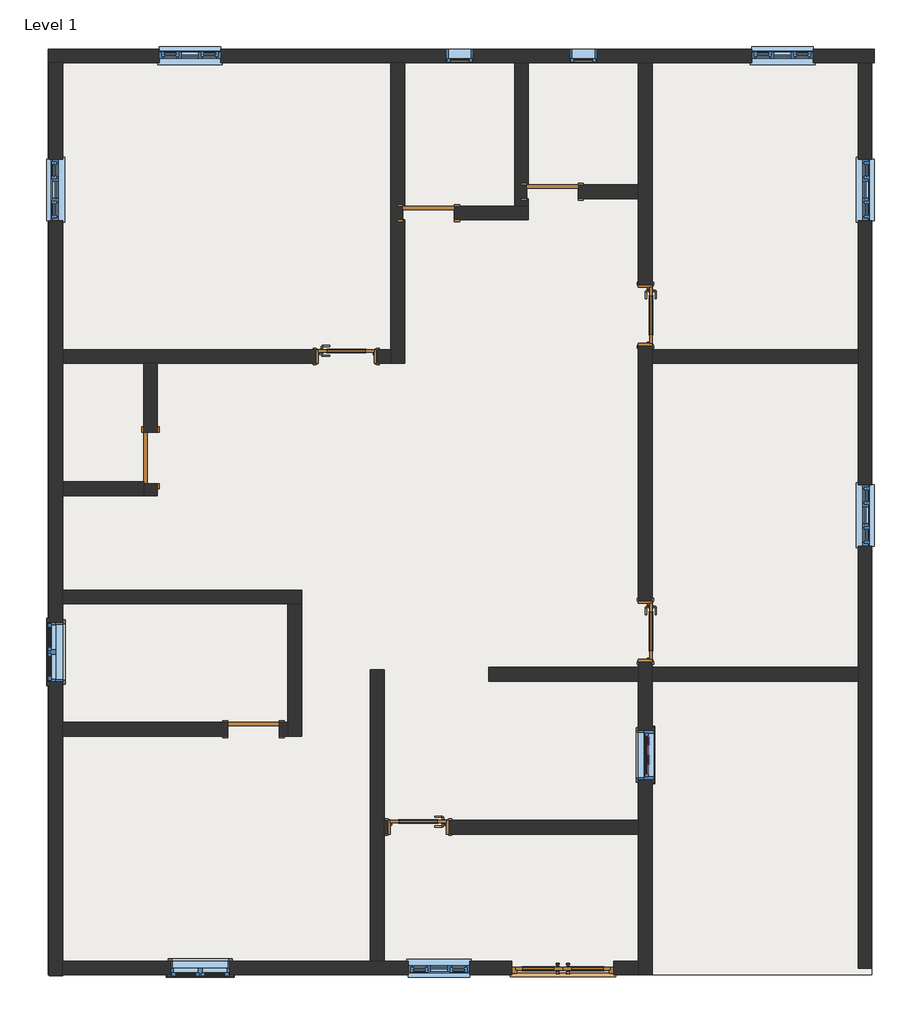
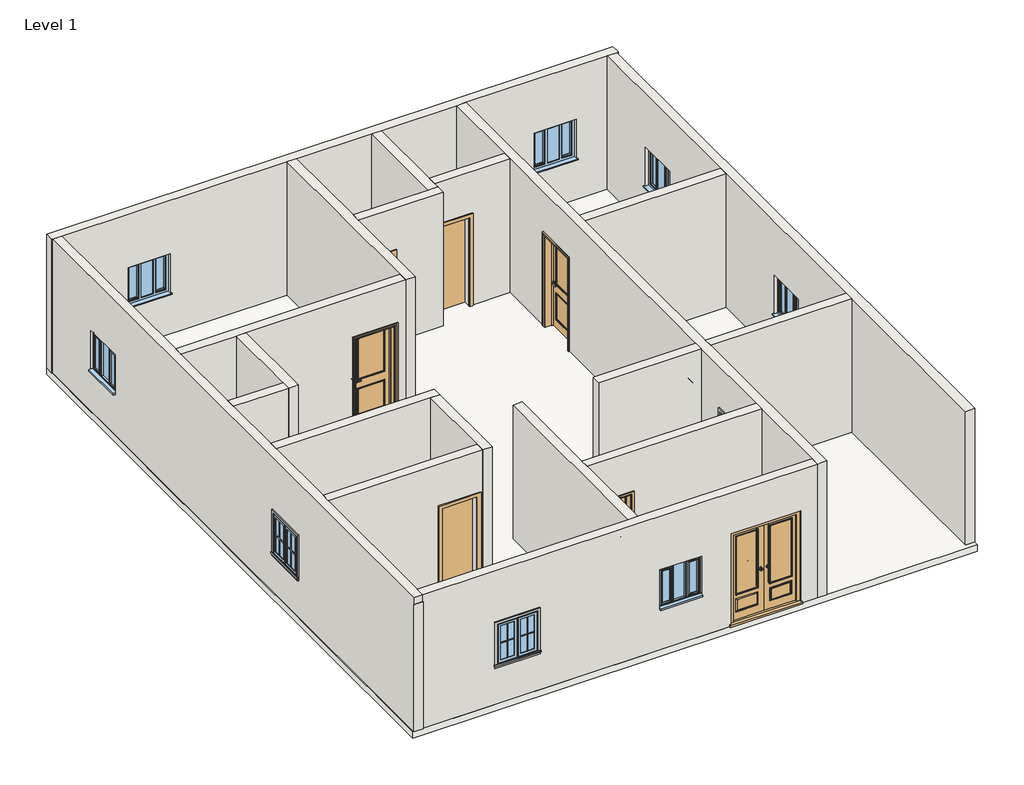
# One storey, incomplete: 19 walls, 12 proxies, 11 windows, 9 doors, 1 slab.
"""IFC4 building model written with IfcOpenShell, lengths in millimetres."""

from ifc_helpers import new_model, si_unit, frame, origin, origin_with_axes, place, context, project, spatial, polyline, outline, extrude, faceted_brep, transform, mapped, element, save
from components import muntin_pattern_2x2_muntin_pattern_2x2_b3fe6957, muntin_pattern_2x2_muntin_pattern_2x2_3e0ecaf2, muntin_pattern_2x2_muntin_pattern_2x2_5f474966, trim_window_exterior_flat_with_sill_41619996, trim_window_exterior_flat_with_sill_68241f6a, trim_window_interior_flat_picture_frame_51c85655, trim_window_interior_flat_picture_frame_d3d93820, doors_extdbl_w_glazing_bars_2_1510x2110mm_e5cd3545, doors_extdbl_w_glazing_bars_2_1510x2110mm_b3535315, doors_intsgl_w_transome_910x2110mm_1071bad6, doors_intsgl_w_transome_910x2110mm_0d7ac49b, door_fadea3f2, door_53b1b562, window_085f26e1, window_c29befe5, window_4d695ea9, windows_tpl_plain_910x910mm_84e79c20

model = new_model("IFC4")

# Units and contexts
model_context = context("Model", 3, world=origin())
ifc_project = project(units=[si_unit("LENGTHUNIT", "METRE", prefix="MILLI")], contexts=[model_context])

# Site, building, storey
site = spatial("IfcSite", under=ifc_project)
building = spatial("IfcBuilding", under=site)
storey = spatial("IfcBuildingStorey", under=building, Name="Level 1", Elevation=0.0)

# Proxies
placement = place(None, origin())
muntin_pattern_2x2_muntin_pattern_2x2_shape = muntin_pattern_2x2_muntin_pattern_2x2_b3fe6957(model_context)
element("IfcBuildingElementProxy", 1, Name="Muntin Pattern_2x2 : Muntin Pattern_2x2", ObjectType="Muntin Pattern_2x2 : Muntin Pattern_2x2", at=placement, inside=storey, context=model_context, shape_type="MappedRepresentation", body=[
    mapped(muntin_pattern_2x2_muntin_pattern_2x2_shape, transform((-4444.3565281, -6259.9254533, 984.25), x_axis=(-1.0, 0.0, 0.0), y_axis=(0.0, -1.0, 0.0), z_axis=(0.0, 0.0, 1.0))),
])
element("IfcBuildingElementProxy", 2, Name="Muntin Pattern_2x2 : Muntin Pattern_2x2", ObjectType="Muntin Pattern_2x2 : Muntin Pattern_2x2", at=placement, inside=storey, context=model_context, shape_type="MappedRepresentation", body=[
    mapped(muntin_pattern_2x2_muntin_pattern_2x2_shape, transform((-6884.3440281, -1708.5629533, 984.25), x_axis=(0.0, 1.0, 0.0), y_axis=(-1.0, 0.0, 0.0), z_axis=(0.0, 0.0, 1.0))),
])
muntin_pattern_2x2_muntin_pattern_2x2_2_shape = muntin_pattern_2x2_muntin_pattern_2x2_3e0ecaf2(model_context)
element("IfcBuildingElementProxy", 3, Name="Muntin Pattern_2x2 : Muntin Pattern_2x2", ObjectType="Muntin Pattern_2x2 : Muntin Pattern_2x2", at=placement, inside=storey, context=model_context, shape_type="MappedRepresentation", body=[
    mapped(muntin_pattern_2x2_muntin_pattern_2x2_2_shape, transform((-4872.9815281, -6259.9254533, 984.25), x_axis=(1.0, 0.0, 0.0), y_axis=(0.0, 1.0, 0.0), z_axis=(0.0, 0.0, 1.0))),
])
element("IfcBuildingElementProxy", 4, Name="Muntin Pattern_2x2 : Muntin Pattern_2x2", ObjectType="Muntin Pattern_2x2 : Muntin Pattern_2x2", at=placement, inside=storey, context=model_context, shape_type="MappedRepresentation", body=[
    mapped(muntin_pattern_2x2_muntin_pattern_2x2_2_shape, transform((-6884.3440281, -1279.9379533, 984.25), x_axis=(0.0, -1.0, 0.0), y_axis=(1.0, 0.0, 0.0), z_axis=(0.0, 0.0, 1.0))),
])
muntin_pattern_2x2_muntin_pattern_2x2_3_shape = muntin_pattern_2x2_muntin_pattern_2x2_5f474966(model_context)
element("IfcBuildingElementProxy", 5, Name="Muntin Pattern_2x2 : Muntin Pattern_2x2", ObjectType="Muntin Pattern_2x2 : Muntin Pattern_2x2", at=placement, inside=storey, context=model_context, shape_type="MappedRepresentation", body=[
    mapped(muntin_pattern_2x2_muntin_pattern_2x2_3_shape, transform((1989.809459, -3018.2504533, 1520.825), x_axis=(0.0, -1.0, 0.0), y_axis=(1.0, 0.0, 0.0), z_axis=(0.0, 0.0, 1.0))),
])
element("IfcBuildingElementProxy", 6, Name="Muntin Pattern_2x2 : Muntin Pattern_2x2", ObjectType="Muntin Pattern_2x2 : Muntin Pattern_2x2", at=placement, inside=storey, context=model_context, shape_type="MappedRepresentation", body=[
    mapped(muntin_pattern_2x2_muntin_pattern_2x2_3_shape, transform((1945.359459, -3018.2504533, 990.6), x_axis=(0.0, -1.0, 0.0), y_axis=(1.0, 0.0, 0.0), z_axis=(0.0, 0.0, 1.0))),
])
trim_window_exterior_flat_with_sill_shape = trim_window_exterior_flat_with_sill_41619996(model_context)
element("IfcBuildingElementProxy", 7, Name="Trim-Window-Exterior-Flat : with Sill", ObjectType="Trim-Window-Exterior-Flat : with Sill", at=placement, inside=storey, context=model_context, shape_type="MappedRepresentation", body=[
    mapped(trim_window_exterior_flat_with_sill_shape, transform((-4658.6690281, -6269.4504533, 1828.8), x_axis=(1.0, 0.0, 0.0), y_axis=(0.0, 0.0, 1.0), z_axis=(0.0, -1.0, 0.0))),
])
element("IfcBuildingElementProxy", 8, Name="Trim-Window-Exterior-Flat : with Sill", ObjectType="Trim-Window-Exterior-Flat : with Sill", at=placement, inside=storey, context=model_context, shape_type="MappedRepresentation", body=[
    mapped(trim_window_exterior_flat_with_sill_shape, transform((-6893.8690281, -1494.2504533, 1828.8), x_axis=(0.0, -1.0, 0.0), y_axis=(0.0, 0.0, 1.0), z_axis=(-1.0, 0.0, 0.0))),
])
trim_window_exterior_flat_with_sill_2_shape = trim_window_exterior_flat_with_sill_68241f6a(model_context)
element("IfcBuildingElementProxy", 9, Name="Trim-Window-Exterior-Flat : with Sill", ObjectType="Trim-Window-Exterior-Flat : with Sill", at=placement, inside=storey, context=model_context, shape_type="MappedRepresentation", body=[
    mapped(trim_window_exterior_flat_with_sill_2_shape, transform((2024.734459, -3018.2504533, 2082.8), x_axis=(0.0, 1.0, 0.0), y_axis=(0.0, 0.0, 1.0), z_axis=(1.0, 0.0, 0.0))),
])
trim_window_interior_flat_picture_frame_shape = trim_window_interior_flat_picture_frame_51c85655(model_context)
element("IfcBuildingElementProxy", 10, Name="Trim-Window-Interior-Flat : Picture Frame", ObjectType="Trim-Window-Interior-Flat : Picture Frame", at=placement, inside=storey, context=model_context, shape_type="MappedRepresentation", body=[
    mapped(trim_window_interior_flat_picture_frame_shape, transform((-4658.6690281, -6066.2504533, 1828.8), x_axis=(-1.0, 0.0, 0.0), y_axis=(0.0, 0.0, 1.0), z_axis=(0.0, 1.0, 0.0))),
])
element("IfcBuildingElementProxy", 11, Name="Trim-Window-Interior-Flat : Picture Frame", ObjectType="Trim-Window-Interior-Flat : Picture Frame", at=placement, inside=storey, context=model_context, shape_type="MappedRepresentation", body=[
    mapped(trim_window_interior_flat_picture_frame_shape, transform((-6690.6690281, -1494.2504533, 1828.8), x_axis=(0.0, 1.0, 0.0), y_axis=(0.0, 0.0, 1.0), z_axis=(1.0, 0.0, 0.0))),
])
trim_window_interior_flat_picture_frame_2_shape = trim_window_interior_flat_picture_frame_d3d93820(model_context)
element("IfcBuildingElementProxy", 12, Name="Trim-Window-Interior-Flat : Picture Frame", ObjectType="Trim-Window-Interior-Flat : Picture Frame", at=placement, inside=storey, context=model_context, shape_type="MappedRepresentation", body=[
    mapped(trim_window_interior_flat_picture_frame_2_shape, transform((1821.534459, -3018.2504533, 2082.8), x_axis=(0.0, -1.0, 0.0), y_axis=(0.0, 0.0, 1.0), z_axis=(-1.0, 0.0, 0.0))),
])

# Doors
doors_extdbl_w_glazing_bars_2_1510x2110mm_shape = doors_extdbl_w_glazing_bars_2_1510x2110mm_e5cd3545(model_context)
doors_extdbl_w_glazing_bars_2_1510x2110mm_2_shape = doors_extdbl_w_glazing_bars_2_1510x2110mm_b3535315(model_context)
element("IfcDoor", 13, ObjectType="Doors_ExtDbl_w-Glazing_Bars_2 : 1510x2110mm", at=placement, inside=storey, context=model_context, shape_type="MappedRepresentation", body=[
    mapped(doors_extdbl_w_glazing_bars_2_1510x2110mm_shape, transform((703.934459, -6167.8504533, 0.0), x_axis=(-1.0, 0.0, 0.0), y_axis=(0.0, -1.0, 0.0), z_axis=(0.0, 0.0, 1.0))),
    mapped(doors_extdbl_w_glazing_bars_2_1510x2110mm_2_shape, transform((703.934459, -6167.8504533, 0.0), x_axis=(-1.0, 0.0, 0.0), y_axis=(0.0, -1.0, 0.0), z_axis=(0.0, 0.0, 1.0))),
])
doors_intsgl_w_transome_910x2110mm_shape = doors_intsgl_w_transome_910x2110mm_1071bad6(model_context)
element("IfcDoor", 14, ObjectType="Doors_IntSgl_w-Transome : 910x2110mm", at=placement, inside=storey, context=model_context, shape_type="MappedRepresentation", body=[
    mapped(doors_intsgl_w_transome_910x2110mm_shape, transform((-1432.8690281, -4085.0504533, 0.0), x_axis=(-1.0, 0.0, 0.0), y_axis=(0.0, -1.0, 0.0), z_axis=(0.0, 0.0, 1.0))),
])
doors_intsgl_w_transome_910x2110mm_2_shape = doors_intsgl_w_transome_910x2110mm_0d7ac49b(model_context)
element("IfcDoor", 15, ObjectType="Doors_IntSgl_w-Transome : 910x2110mm", at=placement, inside=storey, context=model_context, shape_type="MappedRepresentation", body=[
    mapped(doors_intsgl_w_transome_910x2110mm_2_shape, transform((-2499.6690281, 2874.5495467, 0.0), x_axis=(1.0, 0.0, 0.0), y_axis=(0.0, 1.0, 0.0), z_axis=(0.0, 0.0, 1.0))),
])
element("IfcDoor", 16, ObjectType="Doors_IntSgl_w-Transome : 910x2110mm", at=placement, inside=storey, context=model_context, shape_type="MappedRepresentation", body=[
    mapped(doors_intsgl_w_transome_910x2110mm_2_shape, transform((1923.134459, 3484.1495467, 0.0), x_axis=(0.0, -1.0, 0.0), y_axis=(1.0, 0.0, 0.0), z_axis=(0.0, 0.0, 1.0))),
])
element("IfcDoor", 17, ObjectType="Doors_IntSgl_w-Transome : 910x2110mm", at=placement, inside=storey, context=model_context, shape_type="MappedRepresentation", body=[
    mapped(doors_intsgl_w_transome_910x2110mm_2_shape, transform((1923.134459, -1189.4504533, 0.0), x_axis=(0.0, -1.0, 0.0), y_axis=(1.0, 0.0, 0.0), z_axis=(0.0, 0.0, 1.0))),
])
door_shape = door_fadea3f2(model_context)
element("IfcDoor", 18, ObjectType="Single-Flush : 30\" x 80\"", at=placement, inside=storey, context=model_context, shape_type="MappedRepresentation", body=[
    mapped(door_shape, transform((-3871.2690281, -2637.2504533, 0.0), x_axis=(1.0, 0.0, 0.0), y_axis=(0.0, 1.0, 0.0), z_axis=(0.0, 0.0, 1.0))),
])
door_2_shape = door_53b1b562(model_context)
element("IfcDoor", 19, ObjectType="Single-Flush : 30\" x 80\"", at=placement, inside=storey, context=model_context, shape_type="MappedRepresentation", body=[
    mapped(door_2_shape, transform((-5395.2690281, 1375.9495467, 0.0), x_axis=(0.0, -1.0, 0.0), y_axis=(1.0, 0.0, 0.0), z_axis=(0.0, 0.0, 1.0))),
])
element("IfcDoor", 20, ObjectType="Single-Flush : 30\" x 80\"", at=placement, inside=storey, context=model_context, shape_type="MappedRepresentation", body=[
    mapped(door_2_shape, transform((-1280.4690281, 4995.4495467, 0.0), x_axis=(-1.0, 0.0, 0.0), y_axis=(0.0, -1.0, 0.0), z_axis=(0.0, 0.0, 1.0))),
])
element("IfcDoor", 21, ObjectType="Single-Flush : 30\" x 80\"", at=placement, inside=storey, context=model_context, shape_type="MappedRepresentation", body=[
    mapped(door_2_shape, transform((548.3309719, 5312.9495467, 0.0), x_axis=(-1.0, 0.0, 0.0), y_axis=(0.0, -1.0, 0.0), z_axis=(0.0, 0.0, 1.0))),
])

# Slab
element("IfcSlab", 22, ObjectType="Generic - 12\"", at=placement, inside=storey, context=model_context, shape_type="SweptSolid", body=[
    extrude(outline(polyline([(5272.7309719, 7421.1495467), (5272.7309719, -6269.4504533), (-6906.5690281, -6269.4504533), (-6906.5690281, 7421.1495467), (5272.7309719, 7421.1495467)])), frame((0.0, 0.0, -152.4), z_axis=(0.0, 0.0, 1.0), x_axis=(1.0, 0.0, 0.0)), (0.0, 0.0, 1.0), 152.4),
])

# Walls
element("IfcWall", 23, ObjectType="4.5\" p", at=placement, inside=storey, context=model_context, shape_type="Brep", body=[
    faceted_brep([(-1839.2690281, 7217.9495467, 0.0), (-1839.2690281, 2976.1495467, 0.0), (-1839.2690281, 2772.9495467, 0.0), (-1839.2690281, 2772.9495467, 3048.0), (-1839.2690281, 2976.1495467, 3048.0), (-1839.2690281, 7217.9495467, 3048.0), (-1636.0690281, 7217.9495467, 3048.0), (-1636.0690281, 5097.0495467, 3048.0), (-1636.0690281, 4893.8495467, 3048.0), (-1636.0690281, 2772.9495467, 3048.0), (-1636.0690281, 2772.9495467, 0.0), (-1636.0690281, 4893.8495467, 0.0), (-1636.0690281, 4893.8495467, 2032.0), (-1636.0690281, 5097.0495467, 2032.0), (-1636.0690281, 5097.0495467, 0.0), (-1636.0690281, 7217.9495467, 0.0), (-1661.4690281, 5097.0495467, 0.0), (-1661.4690281, 4893.8495467, 0.0), (-1661.4690281, 5097.0495467, 2032.0), (-1661.4690281, 4893.8495467, 2032.0)], [[[0, 1, 2, 3, 4, 5]], [[6, 7, 8, 9, 10, 11, 12, 13, 14, 15]], [[2, 1, 0, 15, 14, 16, 17, 11, 10]], [[5, 4, 3, 9, 8, 7, 6]], [[0, 5, 6, 15]], [[3, 2, 10, 9]], [[18, 16, 14, 13]], [[17, 19, 12, 11]], [[19, 18, 13, 12]], [[16, 18, 19, 17]]]),
])
element("IfcWall", 24, ObjectType="4.5\" p", at=placement, inside=storey, context=model_context, shape_type="Brep", body=[
    faceted_brep([(-1839.2690281, 2772.9495467, 3048.0), (-5293.6690281, 2772.9495467, 3048.0), (-5496.8690281, 2772.9495467, 3048.0), (-6690.6690281, 2772.9495467, 3048.0), (-6690.6690281, 2772.9495467, 0.0), (-5496.8690281, 2772.9495467, 0.0), (-5293.6690281, 2772.9495467, 0.0), (-2954.6690281, 2772.9495467, 0.0), (-2954.6690281, 2772.9495467, 2110.0), (-2044.6690281, 2772.9495467, 2110.0), (-2044.6690281, 2772.9495467, 0.0), (-1839.2690281, 2772.9495467, 0.0), (-6690.6690281, 2976.1495467, 3048.0), (-1839.2690281, 2976.1495467, 3048.0), (-1839.2690281, 2976.1495467, 0.0), (-2044.6690281, 2976.1495467, 0.0), (-2044.6690281, 2976.1495467, 2110.0), (-2954.6690281, 2976.1495467, 2110.0), (-2954.6690281, 2976.1495467, 0.0), (-6690.6690281, 2976.1495467, 0.0)], [[[0, 1, 2, 3, 4, 5, 6, 7, 8, 9, 10, 11]], [[12, 13, 14, 15, 16, 17, 18, 19]], [[4, 19, 18, 7, 6, 5]], [[14, 11, 10, 15]], [[3, 2, 1, 0, 13, 12]], [[0, 11, 14, 13]], [[4, 3, 12, 19]], [[9, 16, 15, 10]], [[16, 9, 8, 17]], [[17, 8, 7, 18]]]),
])
element("IfcWall", 25, ObjectType="4.5\" p", at=placement, inside=storey, context=model_context, shape_type="Brep", body=[
    faceted_brep([(-5496.8690281, 994.9495467, 2032.0), (-5496.8690281, 994.9495467, 0.0), (-5496.8690281, 817.1495467, 0.0), (-5496.8690281, 817.1495467, 3048.0), (-5496.8690281, 1020.3495467, 3048.0), (-5496.8690281, 2772.9495467, 3048.0), (-5496.8690281, 2772.9495467, 0.0), (-5496.8690281, 1756.9495467, 0.0), (-5496.8690281, 1756.9495467, 2032.0), (-5293.6690281, 817.1495467, 0.0), (-5293.6690281, 994.9495467, 0.0), (-5293.6690281, 994.9495467, 2032.0), (-5293.6690281, 1756.9495467, 2032.0), (-5293.6690281, 1756.9495467, 0.0), (-5293.6690281, 2772.9495467, 0.0), (-5293.6690281, 2772.9495467, 3048.0), (-5293.6690281, 817.1495467, 3048.0)], [[[0, 1, 2, 3, 4, 5, 6, 7, 8]], [[9, 10, 11, 12, 13, 14, 15, 16]], [[7, 6, 14, 13]], [[2, 1, 10, 9]], [[5, 4, 3, 16, 15]], [[6, 5, 15, 14]], [[3, 2, 9, 16]], [[11, 10, 1, 0]], [[12, 11, 0, 8]], [[13, 12, 8, 7]]]),
])
element("IfcWall", 26, ObjectType="4.5\" p", at=placement, inside=storey, context=model_context, shape_type="Brep", body=[
    faceted_brep([(-6690.6690281, 817.1495467, 0.0), (-5496.8690281, 817.1495467, 0.0), (-5496.8690281, 817.1495467, 3048.0), (-6690.6690281, 817.1495467, 3048.0), (-6690.6690281, 1020.3495467, 0.0), (-6690.6690281, 1020.3495467, 3048.0), (-5496.8690281, 1020.3495467, 3048.0), (-5496.8690281, 1020.3495467, 0.0), (-5496.8690281, 994.9495467, 0.0)], [[[0, 1, 2, 3]], [[4, 5, 6, 7]], [[1, 0, 4, 7, 8]], [[3, 2, 6, 5]], [[2, 1, 8, 7, 6]], [[0, 3, 5, 4]]]),
])
element("IfcWall", 27, ObjectType="4.5\" p", at=placement, inside=storey, context=model_context, shape_type="Brep", body=[
    faceted_brep([(-6690.6690281, -783.0504533, 0.0), (-3363.2690281, -783.0504533, 0.0), (-3160.0690281, -783.0504533, 0.0), (-3160.0690281, -783.0504533, 3048.0), (-3363.2690281, -783.0504533, 3048.0), (-6690.6690281, -783.0504533, 3048.0), (-6690.6690281, -579.8504533, 0.0), (-6690.6690281, -579.8504533, 3048.0), (-3160.0690281, -579.8504533, 3048.0), (-3160.0690281, -579.8504533, 0.0)], [[[0, 1, 2, 3, 4, 5]], [[6, 7, 8, 9]], [[2, 1, 0, 6, 9]], [[5, 4, 3, 8, 7]], [[0, 5, 7, 6]], [[3, 2, 9, 8]]]),
])
element("IfcWall", 28, ObjectType="4.5\" p", at=placement, inside=storey, context=model_context, shape_type="Brep", body=[
    faceted_brep([(-3363.2690281, -783.0504533, 0.0), (-3363.2690281, -2535.6504533, 0.0), (-3363.2690281, -2738.8504533, 0.0), (-3363.2690281, -2738.8504533, 3048.0), (-3363.2690281, -2535.6504533, 3048.0), (-3363.2690281, -783.0504533, 3048.0), (-3160.0690281, -783.0504533, 0.0), (-3160.0690281, -783.0504533, 3048.0), (-3160.0690281, -2738.8504533, 3048.0), (-3160.0690281, -2738.8504533, 0.0)], [[[0, 1, 2, 3, 4, 5]], [[6, 7, 8, 9]], [[2, 1, 0, 6, 9]], [[5, 4, 3, 8, 7]], [[0, 5, 7, 6]], [[3, 2, 9, 8]]]),
])
element("IfcWall", 29, ObjectType="4.5\" p", at=placement, inside=storey, context=model_context, shape_type="SweptSolid", body=[
    extrude(outline(polyline([(2032.0, -3490.2690281), (0.0, -3490.2690281), (0.0, -3363.2690281), (3048.0, -3363.2690281), (3048.0, -6690.6690281), (0.0, -6690.6690281), (0.0, -4252.2690281), (2032.0, -4252.2690281), (2032.0, -3490.2690281)])), frame((0.0, -2738.8504533, 0.0), z_axis=(0.0, 1.0, 0.0), x_axis=(0.0, 0.0, 1.0)), (0.0, 0.0, 1.0), 203.2),
])
element("IfcWall", 30, ObjectType="4.5\" p", at=placement, inside=storey, context=model_context, shape_type="Brep", body=[
    faceted_brep([(192.7309719, 4893.8495467, 3048.0), (-1636.0690281, 4893.8495467, 3048.0), (-1636.0690281, 4893.8495467, 2032.0), (-899.4690281, 4893.8495467, 2032.0), (-899.4690281, 4893.8495467, 0.0), (192.7309719, 4893.8495467, 0.0), (-1636.0690281, 5097.0495467, 3048.0), (-10.4690281, 5097.0495467, 3048.0), (192.7309719, 5097.0495467, 3048.0), (192.7309719, 5097.0495467, 0.0), (-10.4690281, 5097.0495467, 0.0), (-899.4690281, 5097.0495467, 0.0), (-899.4690281, 5097.0495467, 2032.0), (-1636.0690281, 5097.0495467, 2032.0)], [[[0, 1, 2, 3, 4, 5]], [[6, 7, 8, 9, 10, 11, 12, 13]], [[9, 5, 4, 11, 10]], [[1, 0, 8, 7, 6]], [[1, 6, 13, 2]], [[0, 5, 9, 8]], [[12, 3, 2, 13]], [[3, 12, 11, 4]]]),
])
element("IfcWall", 31, ObjectType="4.5\" p", at=placement, inside=storey, context=model_context, shape_type="Brep", body=[
    faceted_brep([(-10.4690281, 7217.9495467, 0.0), (-10.4690281, 5097.0495467, 0.0), (-10.4690281, 5097.0495467, 3048.0), (-10.4690281, 7217.9495467, 3048.0), (192.7309719, 7217.9495467, 3048.0), (192.7309719, 5414.5495467, 3048.0), (192.7309719, 5211.3495467, 3048.0), (192.7309719, 5097.0495467, 3048.0), (192.7309719, 5097.0495467, 0.0), (192.7309719, 5211.3495467, 0.0), (192.7309719, 5211.3495467, 2032.0), (192.7309719, 5414.5495467, 2032.0), (192.7309719, 5414.5495467, 0.0), (192.7309719, 7217.9495467, 0.0), (167.3309719, 5414.5495467, 0.0), (167.3309719, 5211.3495467, 0.0), (167.3309719, 5414.5495467, 2032.0), (167.3309719, 5211.3495467, 2032.0)], [[[0, 1, 2, 3]], [[4, 5, 6, 7, 8, 9, 10, 11, 12, 13]], [[1, 0, 13, 12, 14, 15, 9, 8]], [[3, 2, 7, 6, 5, 4]], [[2, 1, 8, 7]], [[0, 3, 4, 13]], [[16, 14, 12, 11]], [[15, 17, 10, 9]], [[17, 16, 11, 10]], [[14, 16, 17, 15]]]),
])
element("IfcWall", 32, ObjectType="4.5\" p", at=placement, inside=storey, context=model_context, shape_type="Brep", body=[
    faceted_brep([(1821.534459, -6269.4504533, 3048.0), (1821.534459, -6066.2504533, 3048.0), (1821.534459, -4186.6504533, 3048.0), (1821.534459, -3983.4504533, 3048.0), (1821.534459, -1926.0504533, 3048.0), (1821.534459, -1722.8504533, 3048.0), (1821.534459, 5211.3495467, 3048.0), (1821.534459, 5414.5495467, 3048.0), (1821.534459, 7217.9495467, 3048.0), (1821.534459, 7217.9495467, 0.0), (1821.534459, 5414.5495467, 0.0), (1821.534459, 5211.3495467, 0.0), (1821.534459, 3939.1495467, 0.0), (1821.534459, 3939.1495467, 2110.0), (1821.534459, 3029.1495467, 2110.0), (1821.534459, 3029.1495467, 0.0), (1821.534459, -734.4504533, 0.0), (1821.534459, -734.4504533, 2110.0), (1821.534459, -1644.4504533, 2110.0), (1821.534459, -1644.4504533, 0.0), (1821.534459, -1722.8504533, 0.0), (1821.534459, -1926.0504533, 0.0), (1821.534459, -3983.4504533, 0.0), (1821.534459, -4186.6504533, 0.0), (1821.534459, -6066.2504533, 0.0), (1821.534459, -6269.4504533, 0.0), (1821.534459, -2662.6504533, 2082.8), (1821.534459, -3373.8504533, 2082.8), (1821.534459, -3373.8504533, 914.4), (1821.534459, -2662.6504533, 914.4), (2024.734459, 7217.9495467, 3048.0), (2024.734459, 2976.1495467, 3048.0), (2024.734459, 2772.9495467, 3048.0), (2024.734459, -1722.8504533, 3048.0), (2024.734459, -1926.0504533, 3048.0), (2024.734459, -6269.4504533, 3048.0), (2024.734459, -6269.4504533, 0.0), (2024.734459, -1926.0504533, 0.0), (2024.734459, -1722.8504533, 0.0), (2024.734459, -1644.4504533, 0.0), (2024.734459, -1644.4504533, 2110.0), (2024.734459, -734.4504533, 2110.0), (2024.734459, -734.4504533, 0.0), (2024.734459, 2772.9495467, 0.0), (2024.734459, 2976.1495467, 0.0), (2024.734459, 3029.1495467, 0.0), (2024.734459, 3029.1495467, 2110.0), (2024.734459, 3939.1495467, 2110.0), (2024.734459, 3939.1495467, 0.0), (2024.734459, 7217.9495467, 0.0), (2024.734459, -2662.6504533, 2082.8), (2024.734459, -2662.6504533, 914.4), (2024.734459, -3373.8504533, 914.4), (2024.734459, -3373.8504533, 2082.8)], [[[0, 1, 2, 3, 4, 5, 6, 7, 8, 9, 10, 11, 12, 13, 14, 15, 16, 17, 18, 19, 20, 21, 22, 23, 24, 25], [26, 27, 28, 29]], [[30, 31, 32, 33, 34, 35, 36, 37, 38, 39, 40, 41, 42, 43, 44, 45, 46, 47, 48, 49], [50, 51, 52, 53]], [[9, 49, 48, 12, 11, 10]], [[15, 45, 44, 43, 42, 16]], [[36, 25, 24, 23, 22, 21, 20, 19, 39, 38, 37]], [[8, 7, 6, 5, 4, 3, 2, 1, 0, 35, 34, 33, 32, 31, 30]], [[9, 8, 30, 49]], [[14, 46, 45, 15]], [[46, 14, 13, 47]], [[47, 13, 12, 48]], [[18, 40, 39, 19]], [[40, 18, 17, 41]], [[41, 17, 16, 42]], [[0, 25, 36, 35]], [[51, 50, 26, 29]], [[52, 51, 29, 28]], [[53, 52, 28, 27]], [[50, 53, 27, 26]]]),
])
element("IfcWall", 33, ObjectType="4.5\" p", at=placement, inside=storey, context=model_context, shape_type="SweptSolid", body=[
    extrude(outline(polyline([(-391.4690281, -1926.0504533), (-391.4690281, -1722.8504533), (1821.534459, -1722.8504533), (1821.534459, -1926.0504533), (-391.4690281, -1926.0504533)])), origin_with_axes(), (0.0, 0.0, 1.0), 3048.0),
    extrude(outline(polyline([(5069.5309719, -1722.8504533), (5069.5309719, -1926.0504533), (2024.734459, -1926.0504533), (2024.734459, -1722.8504533), (5069.5309719, -1722.8504533)])), origin_with_axes(), (0.0, 0.0, 1.0), 3048.0),
])
element("IfcWall", 34, ObjectType="4.5\" p", at=placement, inside=storey, context=model_context, shape_type="SweptSolid", body=[
    extrude(outline(polyline([(5069.5309719, 2772.9495467), (2024.734459, 2772.9495467), (2024.734459, 2976.1495467), (5069.5309719, 2976.1495467), (5069.5309719, 2772.9495467)])), origin_with_axes(), (0.0, 0.0, 1.0), 3048.0),
])
element("IfcWall", 35, ObjectType="4.5\" p", at=placement, inside=storey, context=model_context, shape_type="SweptSolid", body=[
    extrude(outline(polyline([(3048.0, 1821.534459), (3048.0, 192.7309719), (2032.0, 192.7309719), (2032.0, 929.3309719), (0.0, 929.3309719), (0.0, 1821.534459), (3048.0, 1821.534459)])), frame((0.0, 5211.3495467, 0.0), z_axis=(0.0, 1.0, 0.0), x_axis=(0.0, 0.0, 1.0)), (0.0, 0.0, 1.0), 203.2),
])
element("IfcWall", 36, ObjectType="4.5\" p", at=placement, inside=storey, context=model_context, shape_type="Brep", body=[
    faceted_brep([(-1940.8690281, -6066.2504533, 0.0), (-1940.8690281, -4186.6504533, 0.0), (-1940.8690281, -3983.4504533, 0.0), (-1940.8690281, -1760.9504533, 0.0), (-1940.8690281, -1760.9504533, 3048.0), (-1940.8690281, -3983.4504533, 3048.0), (-1940.8690281, -4186.6504533, 3048.0), (-1940.8690281, -6066.2504533, 3048.0), (-2144.0690281, -6066.2504533, 0.0), (-2144.0690281, -6066.2504533, 3048.0), (-2144.0690281, -1760.9504533, 3048.0), (-2144.0690281, -1760.9504533, 0.0)], [[[0, 1, 2, 3, 4, 5, 6, 7]], [[8, 9, 10, 11]], [[3, 2, 1, 0, 8, 11]], [[4, 3, 11, 10]], [[7, 6, 5, 4, 10, 9]], [[0, 7, 9, 8]]]),
])
element("IfcWall", 37, ObjectType="4.5\" p", at=placement, inside=storey, context=model_context, shape_type="SweptSolid", body=[
    extrude(outline(polyline([(3048.0, 1821.534459), (3048.0, -1940.8690281), (0.0, -1940.8690281), (0.0, -1887.8690281), (2110.0, -1887.8690281), (2110.0, -977.8690281), (0.0, -977.8690281), (0.0, 1821.534459), (3048.0, 1821.534459)])), frame((0.0, -4186.6504533, 0.0), z_axis=(0.0, 1.0, 0.0), x_axis=(0.0, 0.0, 1.0)), (0.0, 0.0, 1.0), 203.2),
])
element("IfcWall", 38, ObjectType="9\"", at=placement, inside=storey, context=model_context, shape_type="Brep", body=[
    faceted_brep([(5069.5309719, 7217.9495467, 0.0), (5069.5309719, 2976.1495467, 0.0), (5069.5309719, 2772.9495467, 0.0), (5069.5309719, -1722.8504533, 0.0), (5069.5309719, -1926.0504533, 0.0), (5069.5309719, -6167.8504533, 0.0), (5069.5309719, -6167.8504533, 3048.0), (5069.5309719, -1926.0504533, 3048.0), (5069.5309719, -1722.8504533, 3048.0), (5069.5309719, 2772.9495467, 3048.0), (5069.5309719, 2976.1495467, 3048.0), (5069.5309719, 7217.9495467, 3048.0), (5069.5309719, 980.0495467, 1824.4), (5069.5309719, 70.0495467, 1824.4), (5069.5309719, 70.0495467, 914.4), (5069.5309719, 980.0495467, 914.4), (5069.5309719, 5793.3495467, 1824.4), (5069.5309719, 4883.3495467, 1824.4), (5069.5309719, 4883.3495467, 914.4), (5069.5309719, 5793.3495467, 914.4), (5272.7309719, 7217.9495467, 0.0), (5272.7309719, 7217.9495467, 3048.0), (5272.7309719, -6167.8504533, 3048.0), (5272.7309719, -6167.8504533, 0.0), (5272.7309719, 980.0495467, 1824.4), (5272.7309719, 980.0495467, 914.4), (5272.7309719, 70.0495467, 914.4), (5272.7309719, 70.0495467, 1824.4), (5272.7309719, 5793.3495467, 1824.4), (5272.7309719, 5793.3495467, 914.4), (5272.7309719, 4883.3495467, 914.4), (5272.7309719, 4883.3495467, 1824.4)], [[[0, 1, 2, 3, 4, 5, 6, 7, 8, 9, 10, 11], [12, 13, 14, 15], [16, 17, 18, 19]], [[20, 21, 22, 23], [24, 25, 26, 27], [28, 29, 30, 31]], [[5, 4, 3, 2, 1, 0, 20, 23]], [[6, 5, 23, 22]], [[11, 10, 9, 8, 7, 6, 22, 21]], [[0, 11, 21, 20]], [[25, 24, 12, 15]], [[26, 25, 15, 14]], [[27, 26, 14, 13]], [[24, 27, 13, 12]], [[29, 28, 16, 19]], [[30, 29, 19, 18]], [[31, 30, 18, 17]], [[28, 31, 17, 16]]]),
])
element("IfcWall", 39, ObjectType="9\" wall", at=placement, inside=storey, context=model_context, shape_type="Brep", body=[
    faceted_brep([(-6906.5690281, 7217.9495467, 0.0), (-6893.8690281, 7217.9495467, 0.0), (-6690.6690281, 7217.9495467, 0.0), (-1839.2690281, 7217.9495467, 0.0), (-1636.0690281, 7217.9495467, 0.0), (-10.4690281, 7217.9495467, 0.0), (192.7309719, 7217.9495467, 0.0), (1821.534459, 7217.9495467, 0.0), (2024.734459, 7217.9495467, 0.0), (5069.5309719, 7217.9495467, 0.0), (5272.7309719, 7217.9495467, 0.0), (5310.8309719, 7217.9495467, 0.0), (5310.8309719, 7217.9495467, 3048.0), (5272.7309719, 7217.9495467, 3048.0), (5069.5309719, 7217.9495467, 3048.0), (2024.734459, 7217.9495467, 3048.0), (1821.534459, 7217.9495467, 3048.0), (192.7309719, 7217.9495467, 3048.0), (-10.4690281, 7217.9495467, 3048.0), (-1636.0690281, 7217.9495467, 3048.0), (-1839.2690281, 7217.9495467, 3048.0), (-6690.6690281, 7217.9495467, 3048.0), (-6893.8690281, 7217.9495467, 3048.0), (-6906.5690281, 7217.9495467, 3048.0), (-5266.0690281, 7217.9495467, 1824.4), (-4356.0690281, 7217.9495467, 1824.4), (-4356.0690281, 7217.9495467, 914.4), (-5266.0690281, 7217.9495467, 914.4), (3496.9309719, 7217.9495467, 1824.4), (4406.9309719, 7217.9495467, 1824.4), (4406.9309719, 7217.9495467, 914.4), (3496.9309719, 7217.9495467, 914.4), (-1026.4690281, 7217.9495467, 1524.0), (-620.0690281, 7217.9495467, 1524.0), (-620.0690281, 7217.9495467, 914.4), (-1026.4690281, 7217.9495467, 914.4), (803.9327155, 7217.9495467, 1524.0), (1210.3327155, 7217.9495467, 1524.0), (1210.3327155, 7217.9495467, 914.4), (803.9327155, 7217.9495467, 914.4), (-6906.5690281, 7421.1495467, 0.0), (-6906.5690281, 7421.1495467, 3048.0), (5310.8309719, 7421.1495467, 3048.0), (5310.8309719, 7421.1495467, 0.0), (-5266.0690281, 7421.1495467, 1824.4), (-5266.0690281, 7421.1495467, 914.4), (-4356.0690281, 7421.1495467, 914.4), (-4356.0690281, 7421.1495467, 1824.4), (3496.9309719, 7421.1495467, 1824.4), (3496.9309719, 7421.1495467, 914.4), (4406.9309719, 7421.1495467, 914.4), (4406.9309719, 7421.1495467, 1824.4), (-1026.4690281, 7421.1495467, 1524.0), (-1026.4690281, 7421.1495467, 914.4), (-620.0690281, 7421.1495467, 914.4), (-620.0690281, 7421.1495467, 1524.0), (803.9327155, 7421.1495467, 1524.0), (803.9327155, 7421.1495467, 914.4), (1210.3327155, 7421.1495467, 914.4), (1210.3327155, 7421.1495467, 1524.0)], [[[0, 1, 2, 3, 4, 5, 6, 7, 8, 9, 10, 11, 12, 13, 14, 15, 16, 17, 18, 19, 20, 21, 22, 23], [24, 25, 26, 27], [28, 29, 30, 31], [32, 33, 34, 35], [36, 37, 38, 39]], [[40, 41, 42, 43], [44, 45, 46, 47], [48, 49, 50, 51], [52, 53, 54, 55], [56, 57, 58, 59]], [[11, 10, 9, 8, 7, 6, 5, 4, 3, 2, 1, 0, 40, 43]], [[12, 11, 43, 42]], [[23, 22, 21, 20, 19, 18, 17, 16, 15, 14, 13, 12, 42, 41]], [[0, 23, 41, 40]], [[45, 44, 24, 27]], [[46, 45, 27, 26]], [[47, 46, 26, 25]], [[44, 47, 25, 24]], [[49, 48, 28, 31]], [[50, 49, 31, 30]], [[51, 50, 30, 29]], [[48, 51, 29, 28]], [[53, 52, 32, 35]], [[54, 53, 35, 34]], [[55, 54, 34, 33]], [[52, 55, 33, 32]], [[57, 56, 36, 39]], [[58, 57, 39, 38]], [[59, 58, 38, 37]], [[56, 59, 37, 36]]]),
])
element("IfcWall", 40, ObjectType="9\" wall", at=placement, inside=storey, context=model_context, shape_type="Brep", body=[
    faceted_brep([(-6893.8690281, 7217.9495467, 0.0), (-6893.8690281, -6282.1504533, 0.0), (-6893.8690281, -6282.1504533, 2895.6), (-6893.8690281, -6269.4504533, 2895.6), (-6893.8690281, -6269.4504533, 3048.0), (-6893.8690281, 7217.9495467, 3048.0), (-6893.8690281, -1062.4504533, 1828.8), (-6893.8690281, -1926.0504533, 1828.8), (-6893.8690281, -1926.0504533, 914.4), (-6893.8690281, -1062.4504533, 914.4), (-6893.8690281, 4883.3495467, 1824.4), (-6893.8690281, 4883.3495467, 914.4), (-6893.8690281, 5793.3495467, 914.4), (-6893.8690281, 5793.3495467, 1824.4), (-6690.6690281, 7217.9495467, 0.0), (-6690.6690281, 7217.9495467, 3048.0), (-6690.6690281, 2976.1495467, 3048.0), (-6690.6690281, 2772.9495467, 3048.0), (-6690.6690281, 1020.3495467, 3048.0), (-6690.6690281, 817.1495467, 3048.0), (-6690.6690281, -579.8504533, 3048.0), (-6690.6690281, -783.0504533, 3048.0), (-6690.6690281, -2535.6504533, 3048.0), (-6690.6690281, -2738.8504533, 3048.0), (-6690.6690281, -6066.2504533, 3048.0), (-6690.6690281, -6269.4504533, 3048.0), (-6690.6690281, -6269.4504533, 2895.6), (-6690.6690281, -6282.1504533, 2895.6), (-6690.6690281, -6282.1504533, 0.0), (-6690.6690281, -6269.4504533, 0.0), (-6690.6690281, -6066.2504533, 0.0), (-6690.6690281, -2738.8504533, 0.0), (-6690.6690281, -2535.6504533, 0.0), (-6690.6690281, -783.0504533, 0.0), (-6690.6690281, -579.8504533, 0.0), (-6690.6690281, 817.1495467, 0.0), (-6690.6690281, 1020.3495467, 0.0), (-6690.6690281, 2772.9495467, 0.0), (-6690.6690281, 2976.1495467, 0.0), (-6690.6690281, -1062.4504533, 1828.8), (-6690.6690281, -1062.4504533, 914.4), (-6690.6690281, -1926.0504533, 914.4), (-6690.6690281, -1926.0504533, 1828.8), (-6690.6690281, 4883.3495467, 1824.4), (-6690.6690281, 5793.3495467, 1824.4), (-6690.6690281, 5793.3495467, 914.4), (-6690.6690281, 4883.3495467, 914.4)], [[[0, 1, 2, 3, 4, 5], [6, 7, 8, 9], [10, 11, 12, 13]], [[14, 15, 16, 17, 18, 19, 20, 21, 22, 23, 24, 25, 26, 27, 28, 29, 30, 31, 32, 33, 34, 35, 36, 37, 38], [39, 40, 41, 42], [43, 44, 45, 46]], [[1, 0, 14, 38, 37, 36, 35, 34, 33, 32, 31, 30, 29, 28]], [[2, 1, 28, 27]], [[0, 5, 15, 14]], [[40, 39, 6, 9]], [[41, 40, 9, 8]], [[42, 41, 8, 7]], [[39, 42, 7, 6]], [[11, 10, 43, 46]], [[12, 11, 46, 45]], [[13, 12, 45, 44]], [[10, 13, 44, 43]], [[5, 4, 25, 24, 23, 22, 21, 20, 19, 18, 17, 16, 15]], [[25, 4, 3, 26]], [[3, 2, 27, 26]]]),
])
element("IfcWall", 41, ObjectType="9\" wall", at=placement, inside=storey, context=model_context, shape_type="Brep", body=[
    faceted_brep([(1821.534459, -6269.4504533, 3048.0), (-6690.6690281, -6269.4504533, 3048.0), (-6690.6690281, -6269.4504533, 2895.6), (-6690.6690281, -6269.4504533, 0.0), (-51.065541, -6269.4504533, 0.0), (-51.065541, -6269.4504533, 2110.0), (1458.934459, -6269.4504533, 2110.0), (1458.934459, -6269.4504533, 0.0), (1821.534459, -6269.4504533, 0.0), (-5090.4690281, -6269.4504533, 1828.8), (-4226.8690281, -6269.4504533, 1828.8), (-4226.8690281, -6269.4504533, 914.4), (-5090.4690281, -6269.4504533, 914.4), (-673.0690281, -6269.4504533, 1824.4), (-673.0690281, -6269.4504533, 914.4), (-1583.0690281, -6269.4504533, 914.4), (-1583.0690281, -6269.4504533, 1824.4), (-6690.6690281, -6066.2504533, 3048.0), (-2144.0690281, -6066.2504533, 3048.0), (-1940.8690281, -6066.2504533, 3048.0), (1821.534459, -6066.2504533, 3048.0), (1821.534459, -6066.2504533, 0.0), (1458.934459, -6066.2504533, 0.0), (1458.934459, -6066.2504533, 2110.0), (-51.065541, -6066.2504533, 2110.0), (-51.065541, -6066.2504533, 0.0), (-1940.8690281, -6066.2504533, 0.0), (-2144.0690281, -6066.2504533, 0.0), (-6690.6690281, -6066.2504533, 0.0), (-5090.4690281, -6066.2504533, 1828.8), (-5090.4690281, -6066.2504533, 914.4), (-4226.8690281, -6066.2504533, 914.4), (-4226.8690281, -6066.2504533, 1828.8), (-673.0690281, -6066.2504533, 1824.4), (-1583.0690281, -6066.2504533, 1824.4), (-1583.0690281, -6066.2504533, 914.4), (-673.0690281, -6066.2504533, 914.4)], [[[0, 1, 2, 3, 4, 5, 6, 7, 8], [9, 10, 11, 12], [13, 14, 15, 16]], [[17, 18, 19, 20, 21, 22, 23, 24, 25, 26, 27, 28], [29, 30, 31, 32], [33, 34, 35, 36]], [[21, 8, 7, 22]], [[3, 28, 27, 26, 25, 4]], [[1, 0, 20, 19, 18, 17]], [[0, 8, 21, 20]], [[3, 2, 1, 17, 28]], [[30, 29, 9, 12]], [[31, 30, 12, 11]], [[32, 31, 11, 10]], [[29, 32, 10, 9]], [[6, 23, 22, 7]], [[23, 6, 5, 24]], [[24, 5, 4, 25]], [[14, 13, 33, 36]], [[15, 14, 36, 35]], [[16, 15, 35, 34]], [[13, 16, 34, 33]]]),
])

# Windows
window_shape = window_085f26e1(model_context)
element("IfcWindow", 42, ObjectType="Fixed : 16\" x 24\"", at=placement, inside=storey, context=model_context, shape_type="MappedRepresentation", body=[
    mapped(window_shape, transform((-861.3690281, 7319.5495467, 0.0), x_axis=(-1.0, 0.0, 0.0), y_axis=(0.0, -1.0, 0.0), z_axis=(0.0, 0.0, 1.0))),
])
element("IfcWindow", 43, ObjectType="Fixed : 16\" x 24\"", at=placement, inside=storey, context=model_context, shape_type="MappedRepresentation", body=[
    mapped(window_shape, transform((969.0327155, 7319.5495467, 0.0), x_axis=(-1.0, 0.0, 0.0), y_axis=(0.0, -1.0, 0.0), z_axis=(0.0, 0.0, 1.0))),
])
window_2_shape = window_c29befe5(model_context)
element("IfcWindow", 44, ObjectType="Window-Casement-Double : 34\" x 36\"", at=placement, inside=storey, context=model_context, shape_type="MappedRepresentation", body=[
    mapped(window_2_shape, transform((-4658.6690281, -6167.8504533, 0.0), x_axis=(-1.0, 0.0, 0.0), y_axis=(0.0, -1.0, 0.0), z_axis=(0.0, 0.0, 1.0))),
])
element("IfcWindow", 45, ObjectType="Window-Casement-Double : 34\" x 36\"", at=placement, inside=storey, context=model_context, shape_type="MappedRepresentation", body=[
    mapped(window_2_shape, transform((-6792.2690281, -1494.2504533, 0.0), x_axis=(0.0, 1.0, 0.0), y_axis=(-1.0, 0.0, 0.0), z_axis=(0.0, 0.0, 1.0))),
])
window_3_shape = window_4d695ea9(model_context)
element("IfcWindow", 46, ObjectType="Window-Double-Hung : 28\" x 46\"", at=placement, inside=storey, context=model_context, shape_type="MappedRepresentation", body=[
    mapped(window_3_shape, transform((1923.134459, -3018.2504533, 0.0), x_axis=(0.0, -1.0, 0.0), y_axis=(1.0, 0.0, 0.0), z_axis=(0.0, 0.0, 1.0))),
])
windows_tpl_plain_910x910mm_shape = windows_tpl_plain_910x910mm_84e79c20(model_context)
element("IfcWindow", 47, ObjectType="Windows_Tpl_Plain : 910x910mm", at=placement, inside=storey, context=model_context, shape_type="MappedRepresentation", body=[
    mapped(windows_tpl_plain_910x910mm_shape, transform((-1554.7356948, -6159.3938855, -285.6), x_axis=(-1.0, 0.0, 0.0), y_axis=(0.0, -1.0, 0.0), z_axis=(0.0, 0.0, 1.0))),
])
element("IfcWindow", 48, ObjectType="Windows_Tpl_Plain : 910x910mm", at=placement, inside=storey, context=model_context, shape_type="MappedRepresentation", body=[
    mapped(windows_tpl_plain_910x910mm_shape, transform((-6783.8124603, 5765.0162133, -285.6), x_axis=(0.0, 1.0, 0.0), y_axis=(-1.0, 0.0, 0.0), z_axis=(0.0, 0.0, 1.0))),
])
element("IfcWindow", 49, ObjectType="Windows_Tpl_Plain : 910x910mm", at=placement, inside=storey, context=model_context, shape_type="MappedRepresentation", body=[
    mapped(windows_tpl_plain_910x910mm_shape, transform((-4384.4023614, 7311.0929788, -285.6), x_axis=(1.0, 0.0, 0.0), y_axis=(0.0, 1.0, 0.0), z_axis=(0.0, 0.0, 1.0))),
])
element("IfcWindow", 50, ObjectType="Windows_Tpl_Plain : 910x910mm", at=placement, inside=storey, context=model_context, shape_type="MappedRepresentation", body=[
    mapped(windows_tpl_plain_910x910mm_shape, transform((4378.5976386, 7311.0929788, -285.6), x_axis=(1.0, 0.0, 0.0), y_axis=(0.0, 1.0, 0.0), z_axis=(0.0, 0.0, 1.0))),
])
element("IfcWindow", 51, ObjectType="Windows_Tpl_Plain : 910x910mm", at=placement, inside=storey, context=model_context, shape_type="MappedRepresentation", body=[
    mapped(windows_tpl_plain_910x910mm_shape, transform((5162.6744041, 98.38288, -285.6), x_axis=(0.0, -1.0, 0.0), y_axis=(1.0, 0.0, 0.0), z_axis=(0.0, 0.0, 1.0))),
])
element("IfcWindow", 52, ObjectType="Windows_Tpl_Plain : 910x910mm", at=placement, inside=storey, context=model_context, shape_type="MappedRepresentation", body=[
    mapped(windows_tpl_plain_910x910mm_shape, transform((5162.6744041, 4911.68288, -285.6), x_axis=(0.0, -1.0, 0.0), y_axis=(1.0, 0.0, 0.0), z_axis=(0.0, 0.0, 1.0))),
])

save(model, "model.ifc")

# Revit data of these elements
# Type "Muntin Pattern_2x2 : Muntin Pattern_2x2"
#   Width [instance default] = 4' - 0"
#   Thickness = 0' - 0 1/2"
#   Height [instance default] = 4' - 0"
#   Distance = 0' - 0 3/4"
#   Interior Material [instance default] = none
#   Exterior Material [instance default] = none
#   Default Elevation = 0
# Type "Trim-Window-Exterior-Flat : with Sill"
#   Trim Width = 0' - 2 1/4"
#   Trim Thickness_Picture Frame = 0' - 1 1/4"
#   Trim Thickness_with Sill = 0' - 0 3/4"
#   Sill Thickness = 0' - 1 1/4"
#   Opening Width [instance default] = 2' - 0"
#   Opening Height [instance default] = 3' - 0"
#   Default Elevation = 4' - 0"
#   Sill = yes
#   Picture Frame = no
#   Trim Material [instance default] = none
# Type "Trim-Window-Interior-Flat : Picture Frame"
#   Trim Thickness_Picture Frame = 0' - 1 1/4"
#   Trim Width = 0' - 2 1/4"
#   Trim Thickness_with Sill = 0' - 0 3/4"
#   Sill Thickness = 0' - 1 1/4"
#   Opening Width [instance default] = 2' - 0"
#   Opening Height [instance default] = 3' - 0"
#   Default Elevation = 4' - 0"
#   Sill = no
#   Picture Frame = yes
#   Trim Material [instance default] = none
# Type "Doors_ExtDbl_w-Glazing_Bars_2 : 1510x2110mm"
#   Type Mark = "15"
#   Type Comments = "External Double"
#   Operation = "DoubleDoorSingleSwing"
#   Construction Type Id = "GSP4R"
#   Keynote = "L20"
#   Analytic Construction = "1/8 in Pilkington single glazing"
#   Wrap Layers (Int) from Ext = 0' - 6.98819"
#   Wrap Layers (Ext) from Ext = 0' - 4.03543"
#   Visual Light Transmittance = 0.9
#   Top of Intermediate Rail = 1' - 10.6378"
#   Thickness = 0' - 1.73228"
#   Stile Shutting = 0' - 4.92126"
#   Stile - Top Rail = 0' - 3.93701"
#   Stile - Lock Rail = 0' - 3.93701"
#   Stile - Hanging = 0' - 3.93701"
#   Stile - Bottom Rail = 0' - 6.88976"
#   Solar Heat Gain Coefficient = 0.78
#   Rough Width = 4' - 11.44882"
#   Rough Height = 6' - 11.07087"
#   O/A Frame Width = 0' - 2.51969"
#   Heat Transfer Coefficient (U) = 0.6496 BTU/(h·ft²·°F)
#   Handle Z Distance = 3' - 5.33858"
#   Glazing Thickness = 0' - 0.94488"
#   Glazing Bar Thickness = 0' - 0.7874"
#   FrameWidth = 0' - 1.65354"
#   FrameOffset - External = 0' - 0.98425"
#   FrameDepth = 0' - 3.50394"
#   Door Panel Width = 2' - 3.6378"
#   Door Panel Thickness = 0' - 1.73228"
#   Door Panel Height = 6' - 6.74016"
#   Cill Thickness = 0' - 2.14567"
#   Cill Projection = 0' - 1.1811"
#   Handle X Distance = 0' - 2.95276"
#   Height = 6' - 11.07087"
#   Structural Tolerance = 0' - 0.25591"
#   Tolerance = 0' - 0.11811"
#   Undercut = 0' - 0.15748"
#   Width = 4' - 11.44882"
#   Cill Extension = 0' - 0.98425"
#   Cavity Closer Width = 0' - 1.9685"
#   Cavity Closer Offset from Ext = 0' - 4.03543"
#   Cavity Closer Depth = 0' - 3.34646"
#   Vis - Ironmongery = yes
#   Vis - Glazing Bars = yes
#   Vis - Cavity Closers = yes
#   Define Thermal Properties by = 1
#   Function = 1
#   Material Glazing Bars = Door - Panel
#   Material Glass = Door - Glazing
#   Material Door = Door - Panel
#   Material Frame = Door - Frame/Mullion
#   Material Ironmongery = Door - Handle
#   Wall Closure = (empty or 0)
#   Assembly Code = ""
# Type "Doors_IntSgl_w-Transome : 910x2110mm"
#   Type Mark = "11"
#   Type Comments = "Internal Single"
#   Construction Type Id = "SGL"
#   Manufacturer = "Revit"
#   Keynote = "L20"
#   Description = "Internal Single Door"
#   Analytic Construction = "Large single-glazed windows"
#   Visual Light Transmittance = 0.9
#   UnderCut = 0' - 0.31496"
#   Top of Lock Rail = 3' - 3.37008"
#   Tolerance = 0' - 0.07874"
#   Thickness = 0' - 1.49606"
#   Structural Tolerance = 0' - 0.31496"
#   StopDepth = 0' - 1.25984"
#   Stop Thickness = 0' - 0.74803"
#   Stile Top Rail = 0' - 4.92126"
#   Stile Shutting = 0' - 4.92126"
#   Stile Lock Rail = 0' - 7.87402"
#   Stile Hanging = 0' - 4.92126"
#   Stile Bottom Rail = 0' - 7.87402"
#   Solar Heat Gain Coefficient = 0.86
#   Rough Width = 2' - 11.82677"
#   Rough Height = 6' - 11.07087"
#   Height to Top Lock Rail = 3' - 3.37008"
#   Heat Transfer Coefficient (U) = 0.979472 BTU/(h·ft²·°F)
#   Handle Z Distance = 3' - 3.37008"
#   Handle X Distance = 0' - 1.9685"
#   Frame Thickness = 0' - 1.25984"
#   Door Panel Width = 2' - 8.51969"
#   Door Panel Thickness = 0' - 1.49606"
#   Door Panel Offset = 0' - 0"
#   Height = 6' - 11.07087"
#   Width = 2' - 11.82677"
#   Door Panel Height = 6' - 9.10236"
#   Architrave Setback = 0' - 0.19685"
#   Vis - Ironmongery = yes
#   Define Thermal Properties by = 1
#   Material Ironmongery = Door - Handle
#   Material Glass = Door - Glazing
#   Material Frame = Door - Frame/Mullion
#   Material Door = Door - Panel
#   Material Beading = Door - Panel
#   Material Architrave = Door - Architrave
#   Function = (empty or 0)
#   Wall Closure = (empty or 0)
# Type "Single-Flush : 30\" x 80\""
#   Type Mark = "5"
#   Construction Type Id = "MDOOR"
#   Assembly Code = "C1020"
#   Analytic Construction = "Metal"
#   Thickness = 0' - 2"
#   Heat Transfer Coefficient (U) = 0.651978 BTU/(h·ft²·°F)
#   Height = 6' - 8"
#   Trim Projection Ext = 0' - 1"
#   Trim Projection Int = 0' - 1"
#   Trim Width = 0' - 3"
#   Width = 2' - 6"
#   Define Thermal Properties by = 1
#   Define Thermal Properties by = 1
#   Door Material = Door - Panel
#   Frame Material = Door - Frame
#   Visual Light Transmittance = 0
#   Solar Heat Gain Coefficient = 0
#   Function = (empty or 0)
#   Wall Closure = (empty or 0)
# Type "Generic - 12\""
#   Assembly Code = "B1010"
#   Function = 0
#   Layers, outside or top first: 0' - 6" no material (function 1)
# Type "4.5\" p"
#   Assembly Code = "B2010"
#   Layers, outside or top first: 0' - 8" no material (function 1)
# Type "9\""
#   Assembly Code = "B2010"
#   Layers, outside or top first: 0' - 8" no material (function 1)
# Type "9\" wall"
#   Assembly Code = "B2010"
#   Layers, outside or top first: 0' - 8" no material (function 1)
# Type "Fixed : 16\" x 24\""
#   Type Mark = "4"
#   Construction Type Id = "GSP4R"
#   Assembly Code = "B2020100"
#   Analytic Construction = "1/8 in Pilkington single glazing"
#   Visual Light Transmittance = 0.9
#   Solar Heat Gain Coefficient = 0.78
#   Heat Transfer Coefficient (U) = 0.6496 BTU/(h·ft²·°F)
#   Height = 2' - 0"
#   Default Sill Height = 3' - 0"
#   Width = 1' - 4"
#   Window Inset = 0' - 0 3/4"
#   Define Thermal Properties by = 1
#   Define Thermal Properties by = 1
#   Glass Pane Material = Glass
#   Sash Material = Sash
#   Wall Closure = (empty or 0)
# Type "Window-Casement-Double : 34\" x 36\""
#   Type Mark = "14"
#   Fire Rating = "0.5h"
#   Assembly Code = "B2020100"
#   Analytic Construction = "Double glazing - domestic"
#   Frame Extension [instance default] = 0' - 0 1/4"
#   Window Inset [instance default] = 0' - 0"
#   Wall Thickness [instance default] = 0' - 6"
#   Interior Wall Closure [instance default] = 0' - 2 1/4"
#   Half Width = 1' - 5"
#   Visual Light Transmittance = 0.81
#   Thermal Resistance (R) = 1.8146 (h·ft²·°F)/BTU
#   Solar Heat Gain Coefficient = 0.76
#   Rough Width = 2' - 10 1/2"
#   Rough Height = 3' - 0 1/2"
#   Height = 3' - 0"
#   Heat Transfer Coefficient (U) = 0.5511 BTU/(h·ft²·°F)
#   Exterior Wall Closure [instance default] = 0' - 1 1/4"
#   Extension Jamb [instance default] = 0' - 2 1/4"
#   Default Sill Height = 3' - 0"
#   Width = 2' - 10"
#   Define Thermal Properties by = 0
#   Muntin Visibility = yes
#   Interior Trim Visibility [instance default] = yes
#   Exterior Trim Visibility [instance default] = yes
#   Extension Jamb Visibility [instance default] = yes
#   Interior Trim Material = Wood - Stained
#   Muntin Pattern = Muntin Pattern_2x2 : Muntin Pattern_2x2
#   Interior Trim = Trim-Window-Interior-Flat : Picture Frame
#   Interior Frame Material = Wood - Stained
#   Glass Panel Material = Glass
#   Exterior Trim Material = Clad - White
#   Exterior Trim = Trim-Window-Exterior-Flat : with Sill
#   Exterior Frame Material = Clad - White
#   Wall Closure = (empty or 0)
# Type "Window-Double-Hung : 28\" x 46\""
#   Type Mark = "12"
#   Fire Rating = "0.5h"
#   Construction Type Id = "DG-DR"
#   Assembly Code = "B2020100"
#   Analytic Construction = "Double glazing - domestic"
#   Wall Thickness [instance default] = 0' - 6"
#   Window Inset [instance default] = 0' - 0"
#   Visual Light Transmittance = 0.81
#   Thermal Resistance (R) = 1.8146 (h·ft²·°F)/BTU
#   Solar Heat Gain Coefficient = 0.76
#   Muntin Width = 1' - 10"
#   Muntin Height = 1' - 7 1/8"
#   Interior Wall Closure [instance default] = 0' - 1 1/2"
#   Rough Width = 2' - 4 1/2"
#   Rough Height = 3' - 10 1/2"
#   Frame Extension [instance default] = 0' - 1 1/4"
#   Exterior Wall Closure [instance default] = 0' - 0 1/2"
#   Extension Jamb [instance default] = 0' - 1 1/2"
#   Heat Transfer Coefficient (U) = 0.5511 BTU/(h·ft²·°F)
#   Height = 3' - 10"
#   Width = 2' - 4"
#   Define Thermal Properties by = 1
#   Top Muntin Visibility = yes
#   Indicator Visibility [instance default] = yes
#   Extension Jamb Visibility [instance default] = yes
#   Interior Trim Visibility [instance default] = yes
#   Exterior Trim Visibility [instance default] = yes
#   Define Thermal Properties by = 1
#   Bottom Muntin Visibility = yes
#   Muntin Pattern = Muntin Pattern_2x2 : Muntin Pattern_2x2
#   Interior Trim Material = Wood - Stained
#   Interior Trim = Trim-Window-Interior-Flat : Picture Frame
#   Exterior Trim Material = Clad - White
#   Exterior Trim = Trim-Window-Exterior-Flat : with Sill
#   Glass Panel Material = Glass
#   Exterior Frame Material = Clad - White
#   Interior Frame Material = Wood - Stained
#   Wall Closure = (empty or 0)
# Type "Windows_Tpl_Plain : 910x910mm"
#   Type Mark = "24"
#   Operation = "TriplePanelVertical"
#   Construction Type Id = "GSP4R"
#   Manufacturer = "Revit"
#   Keynote = "L10"
#   Analytic Construction = "1/8 in Pilkington single glazing"
#   Wrap Layers (Ext) from Ext = 0' - 4.03543"
#   Wrap Layers (Int) from Ext = 0' - 6.98819"
#   Window Board Projection = 0' - 0.98425"
#   Window Board Extension = 0' - 0.98425"
#   Visual Light Transmittance = 0.9
#   Solar Heat Gain Coefficient = 0.78
#   Rough Width = 2' - 11.82677"
#   Rough Height = 2' - 11.82677"
#   Height = 2' - 11.82677"
#   Width = 2' - 11.82677"
#   Heat Transfer Coefficient (U) = 0.6496 BTU/(h·ft²·°F)
#   Glazing Thickness = 0' - 0.94488"
#   FrameOffset - External = 0' - 1.9685"
#   Frame Depth = 0' - 2.55906"
#   Default Head Height = 6' - 11.07087"
#   Cill Depth = 0' - 3.44488"
#   Cavity Closer Width = 0' - 1.9685"
#   Cavity Closer Offset from Ext = 0' - 4.03543"
#   Cavity Closer Depth = 0' - 3.34646"
#   Vis - Cavity Closers = yes
#   Define Thermal Properties by = 1
#   Material Trim = Window Frame
#   Material Glass = Glass
#   Material Frame = Window Frame
#   Wall Closure = (empty or 0)
# Elements 1, 2, 3, 4 (IfcBuildingElementProxy, "Muntin Pattern_2x2 : Muntin Pattern_2x2")
#   Width = 0' - 11 5/8"
#   Height = 2' - 6 1/2"
#   Interior Material = Wood - Stained
#   Exterior Material = Clad - White
#   Phase Created = New Construction
#   Materials on its faces: "Clad - White", "Wood - Stained"
# Elements 5, 6 (IfcBuildingElementProxy, "Muntin Pattern_2x2 : Muntin Pattern_2x2")
#   Width = 1' - 10"
#   Height = 1' - 7 1/8"
#   Interior Material = Wood - Stained
#   Exterior Material = Clad - White
#   Phase Created = New Construction
#   Materials on its faces: "Clad - White", "Wood - Stained"
# Elements 7, 8 (IfcBuildingElementProxy, "Trim-Window-Exterior-Flat : with Sill")
#   Opening Width = 2' - 10"
#   Opening Height = 3' - 0"
#   Trim Material = Clad - White
#   Phase Created = New Construction
#   Materials on its faces: "Clad - White"
# Element 9 (IfcBuildingElementProxy, "Trim-Window-Exterior-Flat : with Sill")
#   Opening Width = 2' - 4"
#   Opening Height = 3' - 10"
#   Trim Material = Clad - White
#   Phase Created = New Construction
#   Materials on its faces: "Clad - White"
# Elements 10, 11 (IfcBuildingElementProxy, "Trim-Window-Interior-Flat : Picture Frame")
#   Opening Width = 2' - 10"
#   Opening Height = 3' - 0"
#   Trim Material = Wood - Stained
#   Phase Created = New Construction
#   Materials on its faces: "Wood - Stained"
# Element 12 (IfcBuildingElementProxy, "Trim-Window-Interior-Flat : Picture Frame")
#   Opening Width = 2' - 4"
#   Opening Height = 3' - 10"
#   Trim Material = Wood - Stained
#   Phase Created = New Construction
#   Materials on its faces: "Wood - Stained"
# Element 13 (IfcDoor, "Doors_ExtDbl_w-Glazing_Bars_2 : 1510x2110mm")
#   Phase Created = New Construction
#   Materials on its faces: "Door - Panel", "Door - Handle", "Door - Frame/Mullion", "Door - Glazing"
# Elements 14, 15, 16, 17 (IfcDoor, "Doors_IntSgl_w-Transome : 910x2110mm")
#   Phase Created = New Construction
#   Materials on its faces: "Door - Panel", "Door - Architrave", "Door - Handle", "Door - Frame/Mullion", "Door - Glazing"
# Elements 18, 19, 20, 21 (IfcDoor, "Single-Flush : 30\" x 80\"")
#   Phase Created = New Construction
#   Materials on its faces: "Door - Frame", "Door - Panel"
# Element 22 (IfcSlab, "Generic - 12\"")
#   Height Offset From Level = 0' - 0"
#   Phase Created = New Construction
#   Materials on its faces: "Default Floor"
# Elements 23, 24, 25, 26, 27, 28, 29, 30, 31, 33, 34, 35, 36, 37 (IfcWall, "4.5\" p")
#   Top Offset = 0' - 0"
#   Base Offset = 0' - 0"
#   wall height = 10' - 0"
#   Phase Created = New Construction
#   Base Constraint = Level 1
#   Top Constraint = Level 2
#   Materials on its faces: "Default Wall"
# Element 32 (IfcWall, "4.5\" p")
#   Top Offset = 0' - 0"
#   Base Offset = 0' - 0"
#   wall height = 10' - 0"
#   Phase Created = New Construction
#   Base Constraint = Level 1
#   Top Constraint = Level 2
#   Materials on its faces: "Default Wall", "Render Material 255-0-255"
# Element 38 (IfcWall, "9\"")
#   Top Offset = 0' - 0"
#   Base Offset = 0' - 0"
#   wall height = 10' - 0"
#   Phase Created = New Construction
#   Base Constraint = Level 1
#   Top Constraint = Level 2
#   Materials on its faces: "Default Wall"
# Elements 39, 40 (IfcWall, "9\" wall")
#   Top Offset = 0' - 0"
#   Base Offset = 0' - 0"
#   wall height = 10' - 0"
#   Phase Created = New Construction
#   Base Constraint = Level 1
#   Top Constraint = Level 2
#   Materials on its faces: "Default Wall"
# Element 41 (IfcWall, "9\" wall")
#   Top Offset = 0' - 0"
#   Base Offset = 0' - 0"
#   wall height = 10' - 0"
#   Phase Created = New Construction
#   Base Constraint = Level 1
#   Top Constraint = Level 2
#   Materials on its faces: "Default Wall", "Render Material 255-0-255"
# Element 42 (IfcWindow, "Fixed : 16\" x 24\"")
#   Mark = "9"
#   Phase Created = New Construction
#   Materials on its faces: "Sash", "Glass"
# Element 43 (IfcWindow, "Fixed : 16\" x 24\"")
#   Mark = "10"
#   Phase Created = New Construction
